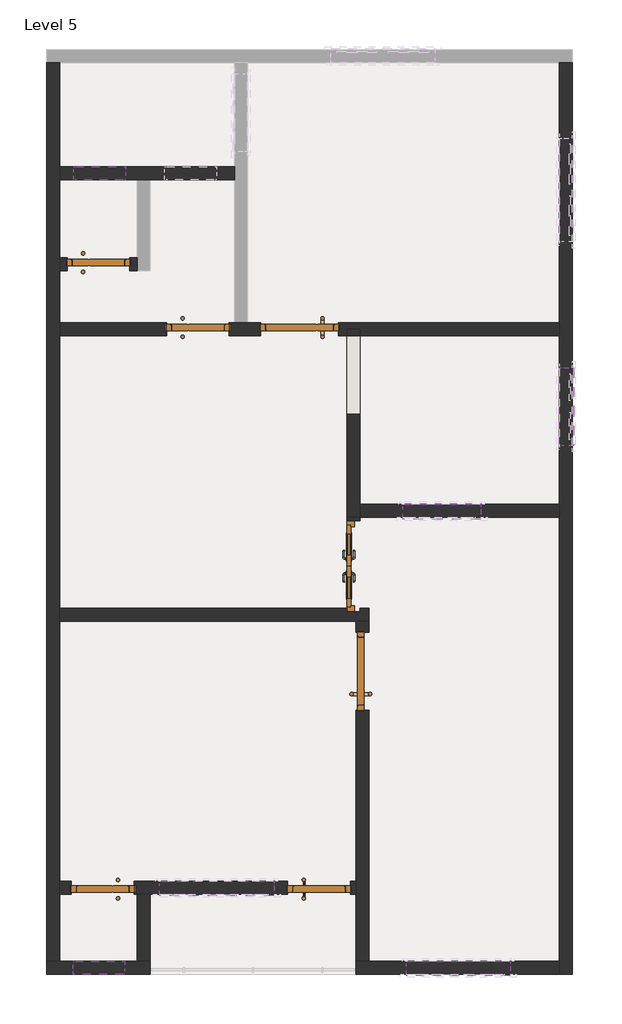
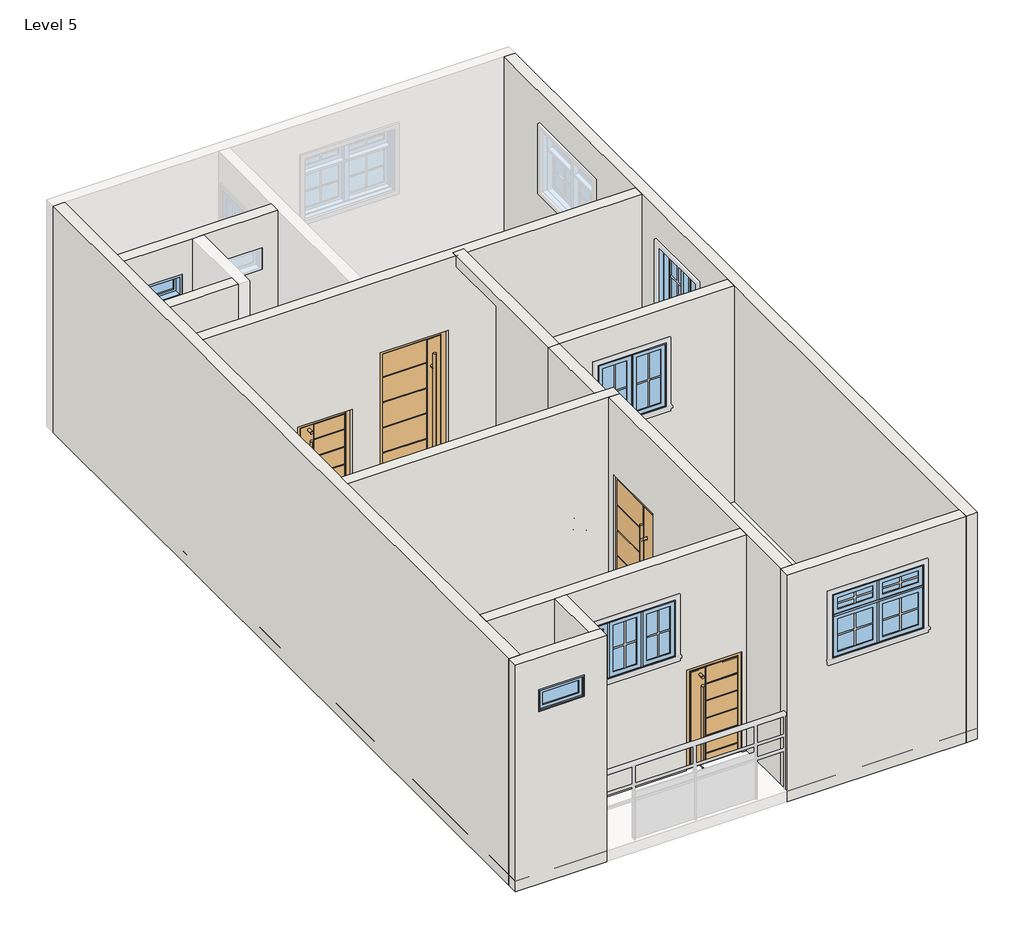
# One storey, part 1 of 2: 14 walls, 7 doors, 6 windows.
"""IFC4 building model written with IfcOpenShell, lengths in millimetres."""

from ifc_helpers import new_model, si_unit, frame, origin, place, context, project, spatial, polyline, outline, extrude, faceted_brep, transform, mapped, element, save
from components import door_9b787682, door_dc81b0c5, door_3_5c4206ef, door_3_79df91aa, door_2576ec39, door_55c03dfd, fixed_2_65c13adb, window_61697a4f, m_window_casement_double_3_e0bd8fa3, m_window_casement_double_awning_double_4_7efa9bbd

model = new_model("IFC4")

# Units and contexts
model_context = context("Model", 3, world=origin())
ifc_project = project(units=[si_unit("LENGTHUNIT", "METRE", prefix="MILLI")], contexts=[model_context])

# Site, building, storey
site = spatial("IfcSite", under=ifc_project)
building = spatial("IfcBuilding", under=site)
storey = spatial("IfcBuildingStorey", under=building, Name="Level 5", Elevation=3810.0)

# Doors
placement = place(None, origin())
door_shape = door_9b787682(model_context)
element("IfcDoor", 1, ObjectType="2'5\"", at=placement, inside=storey, context=model_context, shape_type="MappedRepresentation", body=[
    mapped(door_shape, transform((-22033.2963079, 3049.4742053, 3810.0), x_axis=(1.0, 0.0, 0.0), y_axis=(0.0, 1.0, 0.0), z_axis=(0.0, 0.0, 1.0))),
])
element("IfcDoor", 2, ObjectType="2'5\"", at=placement, inside=storey, context=model_context, shape_type="MappedRepresentation", body=[
    mapped(door_shape, transform((-23201.6963079, 3811.4742053, 3810.0), x_axis=(1.0, 0.0, 0.0), y_axis=(0.0, 1.0, 0.0), z_axis=(0.0, 0.0, 1.0))),
])
element("IfcDoor", 3, ObjectType="2'5\"", at=placement, inside=storey, context=model_context, shape_type="MappedRepresentation", body=[
    mapped(door_shape, transform((-23150.8963079, -3503.7257947, 3810.0), x_axis=(-1.0, 0.0, 0.0), y_axis=(0.0, -1.0, 0.0), z_axis=(0.0, 0.0, 1.0))),
])
door_2_shape = door_dc81b0c5(model_context)
element("IfcDoor", 4, ObjectType="2'5\"", at=placement, inside=storey, context=model_context, shape_type="MappedRepresentation", body=[
    mapped(door_2_shape, transform((-20610.8963079, -3503.7257947, 3856.2445349), x_axis=(1.0, 0.0, 0.0), y_axis=(0.0, 1.0, 0.0), z_axis=(0.0, 0.0, 1.0))),
])
door_3_shape = door_3_5c4206ef(model_context)
element("IfcDoor", 5, ObjectType="3'", at=placement, inside=storey, context=model_context, shape_type="MappedRepresentation", body=[
    mapped(door_3_shape, transform((-20102.8963079, -963.7257947, 3810.0), x_axis=(0.0, 1.0, 0.0), y_axis=(-1.0, 0.0, 0.0), z_axis=(0.0, 0.0, 1.0))),
])
door_3_2_shape = door_3_79df91aa(model_context)
element("IfcDoor", 6, ObjectType="3'", at=placement, inside=storey, context=model_context, shape_type="MappedRepresentation", body=[
    mapped(door_3_2_shape, transform((-20839.4963079, 3049.4742053, 3810.0), x_axis=(-1.0, 0.0, 0.0), y_axis=(0.0, -1.0, 0.0), z_axis=(0.0, 0.0, 1.0))),
])
door_4_shape = door_2576ec39(model_context)
door_5_shape = door_55c03dfd(model_context)
element("IfcDoor", 7, ObjectType="ExtDbl (8) : 3'6\"", at=placement, inside=storey, context=model_context, shape_type="MappedRepresentation", body=[
    mapped(door_4_shape, transform((-20204.4963079, 268.1742053, 3810.0), x_axis=(0.0, -1.0, 0.0), y_axis=(1.0, 0.0, 0.0), z_axis=(0.0, 0.0, 1.0))),
    mapped(door_5_shape, transform((-20204.4963079, 268.1742053, 3810.0), x_axis=(0.0, -1.0, 0.0), y_axis=(1.0, 0.0, 0.0), z_axis=(0.0, 0.0, 1.0))),
])

# Walls
element("IfcWall", 8, ObjectType="Generic - 6\"", at=placement, inside=storey, context=model_context, shape_type="Brep", body=[
    faceted_brep([(-17791.4963079, 6173.6742053, 3810.0), (-17791.4963079, 3125.6742053, 3810.0), (-17791.4963079, 2973.2742053, 3810.0), (-17791.4963079, 992.0742053, 3810.0), (-17791.4963079, 839.6742053, 3810.0), (-17791.4963079, -4367.3257947, 3810.0), (-17791.4963079, -4519.7257947, 3810.0), (-17791.4963079, -4519.7257947, 7010.4), (-17791.4963079, -4367.3257947, 7010.4), (-17791.4963079, 839.6742053, 7010.4), (-17791.4963079, 992.0742053, 7010.4), (-17791.4963079, 2973.2742053, 7010.4), (-17791.4963079, 3125.6742053, 7010.4), (-17791.4963079, 6173.6742053, 7010.4), (-17791.4963079, 4071.8242053, 6538.8), (-17791.4963079, 4071.8242053, 5638.8), (-17791.4963079, 5291.0242053, 5638.8), (-17791.4963079, 5291.0242053, 6538.8), (-17791.4963079, 1682.6367053, 6538.8), (-17791.4963079, 1682.6367053, 5638.8), (-17791.4963079, 2597.0367053, 5638.8), (-17791.4963079, 2597.0367053, 6538.8), (-17639.0963079, 6173.6742053, 3810.0), (-17639.0963079, 6173.6742053, 7010.4), (-17639.0963079, -4519.7257947, 7010.4), (-17639.0963079, -4519.7257947, 3810.0), (-17639.0963079, 4071.8242053, 6538.8), (-17639.0963079, 5291.0242053, 6538.8), (-17639.0963079, 5291.0242053, 5638.8), (-17639.0963079, 4071.8242053, 5638.8), (-17639.0963079, 1682.6367053, 6538.8), (-17639.0963079, 2597.0367053, 6538.8), (-17639.0963079, 2597.0367053, 5638.8), (-17639.0963079, 1682.6367053, 5638.8)], [[[0, 1, 2, 3, 4, 5, 6, 7, 8, 9, 10, 11, 12, 13], [14, 15, 16, 17], [18, 19, 20, 21]], [[22, 23, 24, 25], [26, 27, 28, 29], [30, 31, 32, 33]], [[6, 5, 4, 3, 2, 1, 0, 22, 25]], [[13, 12, 11, 10, 9, 8, 7, 24, 23]], [[0, 13, 23, 22]], [[7, 6, 25, 24]], [[15, 14, 26, 29]], [[16, 15, 29, 28]], [[17, 16, 28, 27]], [[14, 17, 27, 26]], [[19, 18, 30, 33]], [[20, 19, 33, 32]], [[21, 20, 32, 31]], [[18, 21, 31, 30]]]),
])
element("IfcWall", 9, ObjectType="Generic - 6\"", at=placement, inside=storey, context=model_context, shape_type="Brep", body=[
    faceted_brep([(-17791.4963079, -4367.3257947, 3810.0), (-20026.6963079, -4367.3257947, 3810.0), (-20179.0963079, -4367.3257947, 3810.0), (-20179.0963079, -4367.3257947, 7010.4), (-20026.6963079, -4367.3257947, 7010.4), (-17791.4963079, -4367.3257947, 7010.4), (-19585.5697454, -4367.3257947, 6538.8), (-19585.5697454, -4367.3257947, 5638.8), (-18366.3697454, -4367.3257947, 5638.8), (-18366.3697454, -4367.3257947, 6538.8), (-17791.4963079, -4519.7257947, 3810.0), (-17791.4963079, -4519.7257947, 7010.4), (-20179.0963079, -4519.7257947, 7010.4), (-20179.0963079, -4519.7257947, 3810.0), (-19585.5697454, -4519.7257947, 6538.8), (-18366.3697454, -4519.7257947, 6538.8), (-18366.3697454, -4519.7257947, 5638.8), (-19585.5697454, -4519.7257947, 5638.8)], [[[0, 1, 2, 3, 4, 5], [6, 7, 8, 9]], [[10, 11, 12, 13], [14, 15, 16, 17]], [[2, 1, 0, 10, 13]], [[5, 4, 3, 12, 11]], [[0, 5, 11, 10]], [[3, 2, 13, 12]], [[7, 6, 14, 17]], [[8, 7, 17, 16]], [[9, 8, 16, 15]], [[6, 9, 15, 14]]]),
])
element("IfcWall", 10, ObjectType="Generic - 6\"", at=placement, inside=storey, context=model_context, shape_type="Brep", body=[
    faceted_brep([(-23811.2963079, -4519.7257947, 3810.0), (-22592.0963079, -4519.7257947, 3810.0), (-22592.0963079, -4519.7257947, 7010.4), (-23811.2963079, -4519.7257947, 7010.4), (-23500.5431829, -4519.7257947, 6553.2), (-22890.9431829, -4519.7257947, 6553.2), (-22890.9431829, -4519.7257947, 6248.4), (-23500.5431829, -4519.7257947, 6248.4), (-23811.2963079, -4367.3257947, 3810.0), (-23811.2963079, -4367.3257947, 7010.4), (-23658.8963079, -4367.3257947, 7010.4), (-22744.4963079, -4367.3257947, 7010.4), (-22592.0963079, -4367.3257947, 7010.4), (-22592.0963079, -4367.3257947, 3810.0), (-22744.4963079, -4367.3257947, 3810.0), (-23658.8963079, -4367.3257947, 3810.0), (-23500.5431829, -4367.3257947, 6553.2), (-23500.5431829, -4367.3257947, 6248.4), (-22890.9431829, -4367.3257947, 6248.4), (-22890.9431829, -4367.3257947, 6553.2)], [[[0, 1, 2, 3], [4, 5, 6, 7]], [[8, 9, 10, 11, 12, 13, 14, 15], [16, 17, 18, 19]], [[1, 0, 8, 15, 14, 13]], [[3, 2, 12, 11, 10, 9]], [[0, 3, 9, 8]], [[2, 1, 13, 12]], [[17, 16, 4, 7]], [[18, 17, 7, 6]], [[19, 18, 6, 5]], [[16, 19, 5, 4]]]),
])
element("IfcWall", 11, ObjectType="Generic - 6\"", at=placement, inside=storey, context=model_context, shape_type="Brep", body=[
    faceted_brep([(-23658.8963079, -4367.3257947, 3810.0), (-23658.8963079, -3579.9257947, 3810.0), (-23658.8963079, -3427.5257947, 3810.0), (-23658.8963079, -379.5257947, 3810.0), (-23658.8963079, -227.1257947, 3810.0), (-23658.8963079, 2973.2742053, 3810.0), (-23658.8963079, 3125.6742053, 3810.0), (-23658.8963079, 3735.2742053, 3810.0), (-23658.8963079, 3887.6742053, 3810.0), (-23658.8963079, 4802.0742053, 3810.0), (-23658.8963079, 4954.4742053, 3810.0), (-23658.8963079, 6173.6742053, 3810.0), (-23658.8963079, 6173.6742053, 7010.4), (-23658.8963079, 4954.4742053, 7010.4), (-23658.8963079, 4802.0742053, 7010.4), (-23658.8963079, 3887.6742053, 7010.4), (-23658.8963079, 3735.2742053, 7010.4), (-23658.8963079, 3125.6742053, 7010.4), (-23658.8963079, 2973.2742053, 7010.4), (-23658.8963079, -227.1257947, 7010.4), (-23658.8963079, -379.5257947, 7010.4), (-23658.8963079, -3427.5257947, 7010.4), (-23658.8963079, -3579.9257947, 7010.4), (-23658.8963079, -4367.3257947, 7010.4), (-23811.2963079, -4367.3257947, 3810.0), (-23811.2963079, -4367.3257947, 7010.4), (-23811.2963079, 6173.6742053, 7010.4), (-23811.2963079, 6173.6742053, 3810.0)], [[[0, 1, 2, 3, 4, 5, 6, 7, 8, 9, 10, 11, 12, 13, 14, 15, 16, 17, 18, 19, 20, 21, 22, 23]], [[24, 25, 26, 27]], [[11, 10, 9, 8, 7, 6, 5, 4, 3, 2, 1, 0, 24, 27]], [[23, 22, 21, 20, 19, 18, 17, 16, 15, 14, 13, 12, 26, 25]], [[12, 11, 27, 26]], [[0, 23, 25, 24]]]),
])
element("IfcWall", 12, ObjectType="Generic - 6\"", at=placement, inside=storey, context=model_context, shape_type="Brep", body=[
    faceted_brep([(-17791.4963079, 2973.2742053, 7010.4), (-23658.8963079, 2973.2742053, 7010.4), (-23658.8963079, 2973.2742053, 3810.0), (-22401.5963079, 2973.2742053, 3810.0), (-22401.5963079, 2973.2742053, 5334.0), (-21664.9963079, 2973.2742053, 5334.0), (-21664.9963079, 2973.2742053, 3810.0), (-21296.6963079, 2973.2742053, 3810.0), (-21296.6963079, 2973.2742053, 5999.5), (-20382.2963079, 2973.2742053, 5999.5), (-20382.2963079, 2973.2742053, 3810.0), (-17791.4963079, 2973.2742053, 3810.0), (-23658.8963079, 3125.6742053, 7010.4), (-21601.4963079, 3125.6742053, 7010.4), (-21449.0963079, 3125.6742053, 7010.4), (-17791.4963079, 3125.6742053, 7010.4), (-17791.4963079, 3125.6742053, 3810.0), (-20382.2963079, 3125.6742053, 3810.0), (-20382.2963079, 3125.6742053, 5999.5), (-21296.6963079, 3125.6742053, 5999.5), (-21296.6963079, 3125.6742053, 3810.0), (-21449.0963079, 3125.6742053, 3810.0), (-21601.4963079, 3125.6742053, 3810.0), (-21664.9963079, 3125.6742053, 3810.0), (-21664.9963079, 3125.6742053, 5334.0), (-22401.5963079, 3125.6742053, 5334.0), (-22401.5963079, 3125.6742053, 3810.0), (-23658.8963079, 3125.6742053, 3810.0), (-22401.5963079, 3105.6742053, 3810.0), (-22416.5963079, 3105.6742053, 3810.0), (-22416.5963079, 3028.6742053, 3810.0), (-22401.5963079, 3028.6742053, 3810.0), (-20382.2963079, 3028.6742053, 3810.0), (-20367.2963079, 3028.6742053, 3810.0), (-20367.2963079, 3105.6742053, 3810.0), (-20382.2963079, 3105.6742053, 3810.0), (-21296.6963079, 3028.6742053, 3810.0), (-21664.9963079, 3028.6742053, 3810.0), (-21649.9963079, 3028.6742053, 3810.0), (-21649.9963079, 3105.6742053, 3810.0), (-21664.9963079, 3105.6742053, 3810.0), (-21296.6963079, 3105.6742053, 3810.0), (-21311.6963079, 3105.6742053, 3810.0), (-21311.6963079, 3028.6742053, 3810.0), (-21296.6963079, 3105.6742053, 5999.5), (-20382.2963079, 3105.6742053, 5999.5), (-20382.2963079, 3028.6742053, 5999.5), (-21296.6963079, 3028.6742053, 5999.5), (-21311.6963079, 3105.6742053, 6014.5), (-20367.2963079, 3105.6742053, 6014.5), (-20367.2963079, 3028.6742053, 6014.5), (-21311.6963079, 3028.6742053, 6014.5), (-21664.9963079, 3105.6742053, 5334.0), (-22401.5963079, 3105.6742053, 5334.0), (-22401.5963079, 3028.6742053, 5334.0), (-21664.9963079, 3028.6742053, 5334.0), (-22416.5963079, 3105.6742053, 5349.0), (-21649.9963079, 3105.6742053, 5349.0), (-21649.9963079, 3028.6742053, 5349.0), (-22416.5963079, 3028.6742053, 5349.0)], [[[0, 1, 2, 3, 4, 5, 6, 7, 8, 9, 10, 11]], [[12, 13, 14, 15, 16, 17, 18, 19, 20, 21, 22, 23, 24, 25, 26, 27]], [[2, 27, 26, 28, 29, 30, 31, 3]], [[16, 11, 10, 32, 33, 34, 35, 17]], [[36, 7, 6, 37, 38, 39, 40, 23, 22, 21, 20, 41, 42, 43]], [[1, 0, 15, 14, 13, 12]], [[0, 11, 16, 15]], [[2, 1, 12, 27]], [[44, 19, 18, 45]], [[46, 9, 8, 47]], [[19, 44, 41, 20]], [[47, 8, 7, 36]], [[45, 18, 17, 35]], [[9, 46, 32, 10]], [[48, 49, 50, 51]], [[48, 51, 43, 42]], [[46, 47, 36, 43, 51, 50, 33, 32]], [[50, 49, 34, 33]], [[44, 45, 35, 34, 49, 48, 42, 41]], [[24, 52, 53, 25]], [[4, 54, 55, 5]], [[52, 24, 23, 40]], [[5, 55, 37, 6]], [[25, 53, 28, 26]], [[54, 4, 3, 31]], [[56, 57, 58, 59]], [[58, 57, 39, 38]], [[55, 54, 31, 30, 59, 58, 38, 37]], [[56, 59, 30, 29]], [[53, 52, 40, 39, 57, 56, 29, 28]]]),
])
element("IfcWall", 13, ObjectType="Generic - 6\"", at=placement, inside=storey, context=model_context, shape_type="Brep", body=[
    faceted_brep([(-20280.6963079, 3049.4742053, 3810.0), (-20280.6963079, 839.6742053, 3810.0), (-20280.6963079, 839.6742053, 7010.4), (-20280.6963079, 3049.4742053, 7010.4), (-20280.6963079, 2974.7724011, 6858.0), (-20280.6963079, 2050.5574639, 6858.0), (-20280.6963079, 2050.5574639, 4419.6), (-20280.6963079, 2974.7724011, 4419.6), (-20128.2963079, 839.6742053, 3810.0), (-20128.2963079, 992.0742053, 3810.0), (-20128.2963079, 3049.4742053, 3810.0), (-20128.2963079, 3049.4742053, 7010.4), (-20128.2963079, 992.0742053, 7010.4), (-20128.2963079, 839.6742053, 7010.4), (-20128.2963079, 2050.5574639, 6858.0), (-20128.2963079, 2974.7724011, 6858.0), (-20128.2963079, 2974.7724011, 4419.6), (-20128.2963079, 2050.5574639, 4419.6)], [[[0, 1, 2, 3], [4, 5, 6, 7]], [[8, 9, 10, 11, 12, 13], [14, 15, 16, 17]], [[1, 0, 10, 9, 8]], [[3, 2, 13, 12, 11]], [[0, 3, 11, 10]], [[2, 1, 8, 13]], [[4, 15, 14, 5]], [[6, 17, 16, 7]], [[15, 4, 7, 16]], [[5, 14, 17, 6]]]),
])
element("IfcWall", 14, ObjectType="Generic - 6\"", at=placement, inside=storey, context=model_context, shape_type="SweptSolid", body=[
    extrude(outline(polyline([(3810.0, -20128.2963079), (3810.0, -17791.4963079), (7010.4, -17791.4963079), (7010.4, -20128.2963079), (3810.0, -20128.2963079)]), holes=[polyline([(6538.8, -19624.1658391), (6538.8, -18709.7658391), (5638.8, -18709.7658391), (5638.8, -19624.1658391), (6538.8, -19624.1658391)])]), frame((0.0, 839.6742053, 0.0), z_axis=(0.0, 1.0, 0.0), x_axis=(0.0, 0.0, 1.0)), (0.0, 0.0, 1.0), 152.4),
])
element("IfcWall", 15, ObjectType="Generic - 6\"", at=placement, inside=storey, context=model_context, shape_type="Brep", body=[
    faceted_brep([(-23658.8963079, -379.5257947, 3810.0), (-20179.0963079, -379.5257947, 3810.0), (-20026.6963079, -379.5257947, 3810.0), (-20026.6963079, -379.5257947, 7010.4), (-20179.0963079, -379.5257947, 7010.4), (-23658.8963079, -379.5257947, 7010.4), (-23658.8963079, -227.1257947, 7010.4), (-20280.6963079, -227.1257947, 7010.4), (-20128.2963079, -227.1257947, 7010.4), (-20026.6963079, -227.1257947, 7010.4), (-20026.6963079, -227.1257947, 3810.0), (-20128.2963079, -227.1257947, 3810.0), (-20128.2963079, -227.1257947, 5920.0), (-20280.6963079, -227.1257947, 5920.0), (-20280.6963079, -227.1257947, 3810.0), (-23658.8963079, -227.1257947, 3810.0), (-20280.6963079, -265.2257947, 3810.0), (-20128.2963079, -265.2257947, 3810.0), (-20280.6963079, -265.2257947, 5920.0), (-20128.2963079, -265.2257947, 5920.0)], [[[0, 1, 2, 3, 4, 5]], [[6, 7, 8, 9, 10, 11, 12, 13, 14, 15]], [[2, 1, 0, 15, 14, 16, 17, 11, 10]], [[5, 4, 3, 9, 8, 7, 6]], [[0, 5, 6, 15]], [[3, 2, 10, 9]], [[18, 16, 14, 13]], [[17, 19, 12, 11]], [[19, 18, 13, 12]], [[16, 18, 19, 17]]]),
])
element("IfcWall", 16, ObjectType="Generic - 6\"", at=placement, inside=storey, context=model_context, shape_type="Brep", body=[
    faceted_brep([(-20179.0963079, -4367.3257947, 7010.4), (-20179.0963079, -3579.9257947, 7010.4), (-20179.0963079, -3427.5257947, 7010.4), (-20179.0963079, -379.5257947, 7010.4), (-20179.0963079, -379.5257947, 3810.0), (-20179.0963079, -506.5257947, 3810.0), (-20179.0963079, -506.5257947, 5999.5), (-20179.0963079, -1420.9257947, 5999.5), (-20179.0963079, -1420.9257947, 3810.0), (-20179.0963079, -3427.5257947, 3810.0), (-20179.0963079, -3579.9257947, 3810.0), (-20179.0963079, -4367.3257947, 3810.0), (-20026.6963079, -379.5257947, 7010.4), (-20026.6963079, -4367.3257947, 7010.4), (-20026.6963079, -4367.3257947, 3810.0), (-20026.6963079, -1420.9257947, 3810.0), (-20026.6963079, -1420.9257947, 5999.5), (-20026.6963079, -506.5257947, 5999.5), (-20026.6963079, -506.5257947, 3810.0), (-20026.6963079, -379.5257947, 3810.0), (-20082.0963079, -506.5257947, 3810.0), (-20082.0963079, -491.5257947, 3810.0), (-20159.0963079, -491.5257947, 3810.0), (-20159.0963079, -506.5257947, 3810.0), (-20159.0963079, -1420.9257947, 3810.0), (-20159.0963079, -1435.9257947, 3810.0), (-20082.0963079, -1435.9257947, 3810.0), (-20082.0963079, -1420.9257947, 3810.0), (-20159.0963079, -506.5257947, 5999.5), (-20159.0963079, -1420.9257947, 5999.5), (-20082.0963079, -1420.9257947, 5999.5), (-20082.0963079, -506.5257947, 5999.5), (-20159.0963079, -1435.9257947, 6014.5), (-20159.0963079, -491.5257947, 6014.5), (-20082.0963079, -491.5257947, 6014.5), (-20082.0963079, -1435.9257947, 6014.5)], [[[0, 1, 2, 3, 4, 5, 6, 7, 8, 9, 10, 11]], [[12, 13, 14, 15, 16, 17, 18, 19]], [[4, 19, 18, 20, 21, 22, 23, 5]], [[14, 11, 10, 9, 8, 24, 25, 26, 27, 15]], [[3, 2, 1, 0, 13, 12]], [[0, 11, 14, 13]], [[4, 3, 12, 19]], [[6, 28, 29, 7]], [[16, 30, 31, 17]], [[28, 6, 5, 23]], [[17, 31, 20, 18]], [[7, 29, 24, 8]], [[30, 16, 15, 27]], [[32, 33, 34, 35]], [[34, 33, 22, 21]], [[31, 30, 27, 26, 35, 34, 21, 20]], [[32, 35, 26, 25]], [[29, 28, 23, 22, 33, 32, 25, 24]]]),
])
element("IfcWall", 17, ObjectType="Generic - 6\"", at=placement, inside=storey, context=model_context, shape_type="Brep", body=[
    faceted_brep([(-20179.0963079, -3579.9257947, 7010.4), (-22592.0963079, -3579.9257947, 7010.4), (-22744.4963079, -3579.9257947, 7010.4), (-23658.8963079, -3579.9257947, 7010.4), (-23658.8963079, -3579.9257947, 3810.0), (-23519.1963079, -3579.9257947, 3810.0), (-23519.1963079, -3579.9257947, 5334.0), (-22782.5963079, -3579.9257947, 5334.0), (-22782.5963079, -3579.9257947, 3810.0), (-22744.4963079, -3579.9257947, 3810.0), (-22592.0963079, -3579.9257947, 3810.0), (-20179.0963079, -3579.9257947, 3810.0), (-22484.1463079, -3579.9257947, 5638.8), (-22484.1463079, -3579.9257947, 6438.8), (-21137.9463079, -3579.9257947, 6438.8), (-21137.9463079, -3579.9257947, 5638.8), (-20979.1963079, -3579.9257947, 5380.2445349), (-20242.5963079, -3579.9257947, 5380.2445349), (-20242.5963079, -3579.9257947, 3856.2445349), (-20979.1963079, -3579.9257947, 3856.2445349), (-23658.8963079, -3427.5257947, 7010.4), (-20179.0963079, -3427.5257947, 7010.4), (-20179.0963079, -3427.5257947, 3810.0), (-22782.5963079, -3427.5257947, 3810.0), (-22782.5963079, -3427.5257947, 5334.0), (-23519.1963079, -3427.5257947, 5334.0), (-23519.1963079, -3427.5257947, 3810.0), (-23658.8963079, -3427.5257947, 3810.0), (-22484.1463079, -3427.5257947, 6438.8), (-22484.1463079, -3427.5257947, 5638.8), (-21137.9463079, -3427.5257947, 5638.8), (-21137.9463079, -3427.5257947, 6438.8), (-20242.5963079, -3427.5257947, 5380.2445349), (-20979.1963079, -3427.5257947, 5380.2445349), (-20979.1963079, -3427.5257947, 3856.2445349), (-20242.5963079, -3427.5257947, 3856.2445349), (-23519.1963079, -3482.9257947, 3810.0), (-23534.1963079, -3482.9257947, 3810.0), (-23534.1963079, -3559.9257947, 3810.0), (-23519.1963079, -3559.9257947, 3810.0), (-22782.5963079, -3559.9257947, 3810.0), (-22767.5963079, -3559.9257947, 3810.0), (-22767.5963079, -3482.9257947, 3810.0), (-22782.5963079, -3482.9257947, 3810.0), (-20979.1963079, -3559.9257947, 5380.2445349), (-20242.5963079, -3559.9257947, 5380.2445349), (-20242.5963079, -3482.9257947, 5380.2445349), (-20979.1963079, -3482.9257947, 5380.2445349), (-20242.5963079, -3559.9257947, 3856.2445349), (-20242.5963079, -3482.9257947, 3856.2445349), (-20227.5963079, -3559.9257947, 3856.2445349), (-20227.5963079, -3482.9257947, 3856.2445349), (-20979.1963079, -3482.9257947, 3856.2445349), (-20994.1963079, -3482.9257947, 3856.2445349), (-20994.1963079, -3559.9257947, 3856.2445349), (-20979.1963079, -3559.9257947, 3856.2445349), (-20994.1963079, -3559.9257947, 5395.2445349), (-20994.1963079, -3482.9257947, 5395.2445349), (-20227.5963079, -3482.9257947, 5395.2445349), (-20227.5963079, -3559.9257947, 5395.2445349), (-23519.1963079, -3559.9257947, 5334.0), (-22782.5963079, -3559.9257947, 5334.0), (-22782.5963079, -3482.9257947, 5334.0), (-23519.1963079, -3482.9257947, 5334.0), (-22767.5963079, -3559.9257947, 5349.0), (-23534.1963079, -3559.9257947, 5349.0), (-23534.1963079, -3482.9257947, 5349.0), (-22767.5963079, -3482.9257947, 5349.0)], [[[0, 1, 2, 3, 4, 5, 6, 7, 8, 9, 10, 11], [12, 13, 14, 15], [16, 17, 18, 19]], [[20, 21, 22, 23, 24, 25, 26, 27], [28, 29, 30, 31], [32, 33, 34, 35]], [[4, 27, 26, 36, 37, 38, 39, 5]], [[22, 11, 10, 9, 8, 40, 41, 42, 43, 23]], [[3, 2, 1, 0, 21, 20]], [[4, 3, 20, 27]], [[0, 11, 22, 21]], [[29, 28, 13, 12]], [[30, 29, 12, 15]], [[31, 30, 15, 14]], [[28, 31, 14, 13]], [[16, 44, 45, 17]], [[32, 46, 47, 33]], [[17, 45, 48, 18]], [[46, 32, 35, 49]], [[18, 48, 50, 51, 49, 35, 34, 52, 53, 54, 55, 19]], [[44, 16, 19, 55]], [[33, 47, 52, 34]], [[56, 57, 58, 59]], [[51, 50, 59, 58]], [[47, 46, 49, 51, 58, 57, 53, 52]], [[54, 53, 57, 56]], [[45, 44, 55, 54, 56, 59, 50, 48]], [[6, 60, 61, 7]], [[24, 62, 63, 25]], [[60, 6, 5, 39]], [[25, 63, 36, 26]], [[7, 61, 40, 8]], [[62, 24, 23, 43]], [[64, 65, 66, 67]], [[66, 65, 38, 37]], [[63, 62, 43, 42, 67, 66, 37, 36]], [[64, 67, 42, 41]], [[61, 60, 39, 38, 65, 64, 41, 40]]]),
])
element("IfcWall", 18, ObjectType="Generic - 6\"", at=placement, inside=storey, context=model_context, shape_type="SweptSolid", body=[
    extrude(outline(polyline([(-22744.4963079, -4367.3257947), (-22744.4963079, -3579.9257947), (-22592.0963079, -3579.9257947), (-22592.0963079, -4367.3257947), (-22744.4963079, -4367.3257947)])), frame((0.0, 0.0, 3810.0), z_axis=(0.0, 0.0, 1.0), x_axis=(1.0, 0.0, 0.0)), (0.0, 0.0, 1.0), 3200.4),
])
element("IfcWall", 19, ObjectType="Generic - 6\"", at=placement, inside=storey, context=model_context, shape_type="Brep", body=[
    faceted_brep([(-23658.8963079, 4802.0742053, 3810.0), (-22744.4963079, 4802.0742053, 3810.0), (-22592.0963079, 4802.0742053, 3810.0), (-21601.4963079, 4802.0742053, 3810.0), (-21601.4963079, 4802.0742053, 7010.4), (-22592.0963079, 4802.0742053, 7010.4), (-22744.4963079, 4802.0742053, 7010.4), (-23658.8963079, 4802.0742053, 7010.4), (-22880.5252141, 4802.0742053, 6553.2), (-22880.5252141, 4802.0742053, 6248.4), (-23490.1252141, 4802.0742053, 6248.4), (-23490.1252141, 4802.0742053, 6553.2), (-21812.6338079, 4802.0742053, 6553.2), (-21812.6338079, 4802.0742053, 6248.4), (-22422.2338079, 4802.0742053, 6248.4), (-22422.2338079, 4802.0742053, 6553.2), (-23658.8963079, 4954.4742053, 3810.0), (-23658.8963079, 4954.4742053, 7010.4), (-21601.4963079, 4954.4742053, 7010.4), (-21601.4963079, 4954.4742053, 3810.0), (-22880.5252141, 4954.4742053, 6553.2), (-23490.1252141, 4954.4742053, 6553.2), (-23490.1252141, 4954.4742053, 6248.4), (-22880.5252141, 4954.4742053, 6248.4), (-21812.6338079, 4954.4742053, 6553.2), (-22422.2338079, 4954.4742053, 6553.2), (-22422.2338079, 4954.4742053, 6248.4), (-21812.6338079, 4954.4742053, 6248.4)], [[[0, 1, 2, 3, 4, 5, 6, 7], [8, 9, 10, 11], [12, 13, 14, 15]], [[16, 17, 18, 19], [20, 21, 22, 23], [24, 25, 26, 27]], [[3, 2, 1, 0, 16, 19]], [[7, 6, 5, 4, 18, 17]], [[0, 7, 17, 16]], [[4, 3, 19, 18]], [[9, 8, 20, 23]], [[10, 9, 23, 22]], [[11, 10, 22, 21]], [[8, 11, 21, 20]], [[13, 12, 24, 27]], [[14, 13, 27, 26]], [[15, 14, 26, 25]], [[12, 15, 25, 24]]]),
])
element("IfcWall", 20, ObjectType="Generic - 6\"", at=placement, inside=storey, context=model_context, shape_type="Brep", body=[
    faceted_brep([(-22744.4963079, 3735.2742053, 7010.4), (-23658.8963079, 3735.2742053, 7010.4), (-23658.8963079, 3735.2742053, 3810.0), (-23569.9963079, 3735.2742053, 3810.0), (-23569.9963079, 3735.2742053, 5334.0), (-22833.3963079, 3735.2742053, 5334.0), (-22833.3963079, 3735.2742053, 3810.0), (-22744.4963079, 3735.2742053, 3810.0), (-23658.8963079, 3887.6742053, 7010.4), (-22744.4963079, 3887.6742053, 7010.4), (-22744.4963079, 3887.6742053, 3810.0), (-22833.3963079, 3887.6742053, 3810.0), (-22833.3963079, 3887.6742053, 5334.0), (-23569.9963079, 3887.6742053, 5334.0), (-23569.9963079, 3887.6742053, 3810.0), (-23658.8963079, 3887.6742053, 3810.0), (-23569.9963079, 3867.6742053, 3810.0), (-23584.9963079, 3867.6742053, 3810.0), (-23584.9963079, 3790.6742053, 3810.0), (-23569.9963079, 3790.6742053, 3810.0), (-22833.3963079, 3790.6742053, 3810.0), (-22818.3963079, 3790.6742053, 3810.0), (-22818.3963079, 3867.6742053, 3810.0), (-22833.3963079, 3867.6742053, 3810.0), (-22833.3963079, 3867.6742053, 5334.0), (-23569.9963079, 3867.6742053, 5334.0), (-23569.9963079, 3790.6742053, 5334.0), (-22833.3963079, 3790.6742053, 5334.0), (-23584.9963079, 3867.6742053, 5349.0), (-22818.3963079, 3867.6742053, 5349.0), (-22818.3963079, 3790.6742053, 5349.0), (-23584.9963079, 3790.6742053, 5349.0)], [[[0, 1, 2, 3, 4, 5, 6, 7]], [[8, 9, 10, 11, 12, 13, 14, 15]], [[2, 15, 14, 16, 17, 18, 19, 3]], [[10, 7, 6, 20, 21, 22, 23, 11]], [[1, 0, 9, 8]], [[0, 7, 10, 9]], [[2, 1, 8, 15]], [[12, 24, 25, 13]], [[4, 26, 27, 5]], [[24, 12, 11, 23]], [[5, 27, 20, 6]], [[13, 25, 16, 14]], [[26, 4, 3, 19]], [[28, 29, 30, 31]], [[30, 29, 22, 21]], [[27, 26, 19, 18, 31, 30, 21, 20]], [[28, 31, 18, 17]], [[25, 24, 23, 22, 29, 28, 17, 16]]]),
])
element("IfcWall", 21, ObjectType="Generic - 6\"", at=placement, inside=storey, context=model_context, shape_type="SweptSolid", body=[
    extrude(outline(polyline([(-227.1257947, 7010.4), (839.6742053, 7010.4), (839.6742053, 3810.0), (801.5742053, 3810.0), (801.5742053, 5920.0), (-227.1257947, 5920.0), (-227.1257947, 7010.4)])), frame((-20280.6963079, 0.0, 0.0), z_axis=(1.0, 0.0, 0.0), x_axis=(0.0, 1.0, 0.0)), (0.0, 0.0, 1.0), 152.4),
])

# Windows
fixed_2_shape = fixed_2_65c13adb(model_context)
element("IfcWindow", 22, ObjectType="Fixed : 2'", at=placement, inside=storey, context=model_context, shape_type="MappedRepresentation", body=[
    mapped(fixed_2_shape, transform((-23233.8431829, -4443.5257947, 5334.0), x_axis=(-1.0, 0.0, 0.0), y_axis=(0.0, -1.0, 0.0), z_axis=(0.0, 0.0, 1.0))),
])
element("IfcWindow", 23, ObjectType="Fixed : 2'", at=placement, inside=storey, context=model_context, shape_type="MappedRepresentation", body=[
    mapped(fixed_2_shape, transform((-23147.2252141, 4878.2742053, 5334.0), x_axis=(1.0, 0.0, 0.0), y_axis=(0.0, 1.0, 0.0), z_axis=(0.0, 0.0, 1.0))),
])
window_shape = window_61697a4f(model_context)
element("IfcWindow", 24, ObjectType="M_Window-Awning-Triple-Horizontal : 4'5\"", at=placement, inside=storey, context=model_context, shape_type="MappedRepresentation", body=[
    mapped(window_shape, transform((-21811.0463079, -3503.7257947, 4738.8), x_axis=(-1.0, 0.0, 0.0), y_axis=(0.0, -1.0, 0.0), z_axis=(0.0, 0.0, 1.0))),
])
m_window_casement_double_3_shape = m_window_casement_double_3_e0bd8fa3(model_context)
element("IfcWindow", 25, ObjectType="M_Window-Casement-Double : 3'", at=placement, inside=storey, context=model_context, shape_type="MappedRepresentation", body=[
    mapped(m_window_casement_double_3_shape, transform((-19166.9658391, 915.8742053, 4738.8), x_axis=(-1.0, 0.0, 0.0), y_axis=(0.0, -1.0, 0.0), z_axis=(0.0, 0.0, 1.0))),
])
element("IfcWindow", 26, ObjectType="M_Window-Casement-Double : 3'", at=placement, inside=storey, context=model_context, shape_type="MappedRepresentation", body=[
    mapped(m_window_casement_double_3_shape, transform((-17715.2963079, 2139.8367053, 4738.8), x_axis=(0.0, -1.0, 0.0), y_axis=(1.0, 0.0, 0.0), z_axis=(0.0, 0.0, 1.0))),
])
m_window_casement_double_awning_double_4_shape = m_window_casement_double_awning_double_4_7efa9bbd(model_context)
element("IfcWindow", 27, ObjectType="M_Window-Casement-Double-Awning-Double : 4'", at=placement, inside=storey, context=model_context, shape_type="MappedRepresentation", body=[
    mapped(m_window_casement_double_awning_double_4_shape, transform((-18975.9697454, -4443.5257947, 4738.8), x_axis=(-1.0, 0.0, 0.0), y_axis=(0.0, -1.0, 0.0), z_axis=(0.0, 0.0, 1.0))),
])

save(model, "model.ifc")

# Revit data of these elements
# Type "2'5\""
#   Type Mark = "9"
#   Water resistance = "up to Class E900, EN 12208:2001"
#   Uniclass2015Version = "v1.21"
#   Uniclass2015Reference = "Ss_25_30_20_30"
#   Uniclass2015Description = "Frame and door leaf system"
#   URL = "www.aluprof.com"
#   Type IFC Predefined Type = "USERDEFINED"
#   Right-hand / Left-hand door [instance default] = ""
#   Resistance to wind load = "up to Class C5/B5, EN 12210:2001"
#   Insert type = "ST"
#   Hardware [instance default] = ""
#   Product page = "https://aluprof.com/en/architects/offer/window-and-door-systems/panel-doors#visualisation"
#   Operation = "SinglePanelOutwardOpening"
#   Opening type = "Outward"
#   NBSReference = "25-50-20/125"
#   NBSDescription = "Frame and door leaf system"
#   Important = "The actual acceptable construction dimensions are dependent on the selection of profiles and hardware, glazing type, construction weight and the construction’s operating conditions. These should be determined by a suitably qualified person, and using ALUPROF’s calculation software"
#   IfcExportType = "USERDEFINED"
#   IfcExportAs = "IfcDoorType"
#   Handle type [instance default] = ""
#   Manufacturer = "ALUPROF SA"
#   Export Type to IFC As = "IfcDoorType"
#   Door sill type [instance default] = ""
#   Description = "External single-leaf panel door outward opening"
#   Model = "MB-86 ST Panel Door AD07"
#   Content of the recyclate in the material = "69.2%"
#   COBie.Type.WarrantyDurationParts = ""
#   COBie.Type.Name = ""
#   COBie.Type.Manufacturer = "ALUPROF SA"
#   COBie.Space.Name = ""
#   COBie.Floor.Name = ""
#   COBie.Facility.Name = ""
#   COBie.CreatedOn = ""
#   COBie.Component.WarrantyStartDate = ""
#   COBie.Component.Name = "MB-86 ST Panel Door AD07"
#   Burglar resistance = "RC2"
#   Air permeability = "up to Class 4, EN 12207:2001"
#   Width of the active leaf = 2' - 1.17717"
#   Placement in wall = 0' - 0.7874"
#   Thickness = 0' - 3.0315"
#   Height of the opening sash = 4' - 9.44094"
#   Handle Offset = 3' - 5.33858"
#   Rough Height = 5' - 2.40945"
#   Rough Width = 2' - 6.1811"
#   Height = 5' - 0"
#   Width = 2' - 5"
#   Construction depth = 0' - 3.0315"
#   Clear opening width = 1' - 8.94882"
#   Clear opening height = 4' - 8.47638"
#   Height of the array = 0' - 9.08136"
#   Schedule No. [instance default] = 1
#   Handrail [instance default] = yes
#   IsExternal = yes
#   Handle [instance default] = no
#   Door closer [instance default] = no
#   Function = 1
#   COBie.Type = yes
#   COBie = yes
#   Access control [instance default] = no
#   Panel = element 346771
#   Wall Closure = (empty or 0)
# Type "3'"
#   Type Mark = "10"
#   Water resistance = "up to Class E900, EN 12208:2001"
#   Uniclass2015Version = "v1.21"
#   Uniclass2015Reference = "Ss_25_30_20_30"
#   Uniclass2015Description = "Frame and door leaf system"
#   URL = "www.aluprof.com"
#   Type IFC Predefined Type = "USERDEFINED"
#   Right-hand / Left-hand door [instance default] = ""
#   Resistance to wind load = "up to Class C5/B5, EN 12210:2001"
#   Insert type = "ST"
#   Hardware [instance default] = ""
#   Product page = "https://aluprof.com/en/architects/offer/window-and-door-systems/panel-doors#visualisation"
#   Operation = "SinglePanelOutwardOpening"
#   Opening type = "Outward"
#   NBSReference = "25-50-20/125"
#   NBSDescription = "Frame and door leaf system"
#   Important = "The actual acceptable construction dimensions are dependent on the selection of profiles and hardware, glazing type, construction weight and the construction’s operating conditions. These should be determined by a suitably qualified person, and using ALUPROF’s calculation software"
#   IfcExportType = "USERDEFINED"
#   IfcExportAs = "IfcDoorType"
#   Handle type [instance default] = ""
#   Manufacturer = "ALUPROF SA"
#   Export Type to IFC As = "IfcDoorType"
#   Door sill type [instance default] = ""
#   Description = "External single-leaf panel door outward opening"
#   Model = "MB-86 ST Panel Door AD07"
#   Content of the recyclate in the material = "69.2%"
#   COBie.Type.WarrantyDurationParts = ""
#   COBie.Type.Name = ""
#   COBie.Type.Manufacturer = "ALUPROF SA"
#   COBie.Space.Name = ""
#   COBie.Floor.Name = ""
#   COBie.Facility.Name = ""
#   COBie.CreatedOn = ""
#   COBie.Component.WarrantyStartDate = ""
#   COBie.Component.Name = "MB-86 ST Panel Door AD07"
#   Burglar resistance = "RC2"
#   Air permeability = "up to Class 4, EN 12207:2001"
#   Width of the active leaf = 2' - 8.17717"
#   Placement in wall = 0' - 0.7874"
#   Thickness = 0' - 3.0315"
#   Height of the opening sash = 6' - 11.64173"
#   Handle Offset = 3' - 5.33858"
#   Rough Height = 7' - 4.61024"
#   Rough Width = 3' - 1.1811"
#   Height = 7' - 2.20079"
#   Width = 3' - 0"
#   Construction depth = 0' - 3.0315"
#   Clear opening width = 2' - 3.94882"
#   Clear opening height = 6' - 10.67717"
#   Height of the array = 1' - 1.44816"
#   Schedule No. [instance default] = 1
#   Handrail [instance default] = yes
#   IsExternal = yes
#   Handle [instance default] = no
#   Door closer [instance default] = no
#   Function = 1
#   COBie.Type = yes
#   COBie = yes
#   Access control [instance default] = no
#   Panel = element 346771
#   Wall Closure = (empty or 0)
# Type "ExtDbl (8) : 3'6\""
#   Type Mark = "14"
#   Operation = "DoubleDoorSingleSwing"
#   Keynote = "L20"
#   Wrap Layers (Int) from Ext = 0' - 6.98819"
#   Wrap Layers (Ext) from Ext = 0' - 4.03543"
#   Top of Lock Rail = 2' - 11.43307"
#   Thickness = 0' - 1.73228"
#   Stile Shutting = 0' - 4.92126"
#   Stile - Top Rail = 0' - 5.90551"
#   Stile - Lock Rail = 0' - 5.90551"
#   Stile - Hanging = 0' - 3.93701"
#   Stile - Bottom Rail = 0' - 11.81102"
#   Rough Width = 3' - 6"
#   Rough Height = 6' - 11.07087"
#   O/A Frame Width = 0' - 2.51969"
#   Handle Z Distance = 3' - 1.40157"
#   Glazing Thickness = 0' - 0.94488"
#   FrameWidth = 0' - 1.65354"
#   FrameOffset - External = 0' - 2.55906"
#   FrameDepth = 0' - 3.50394"
#   Door Panel Width = 1' - 6.91339"
#   Door Panel Thickness = 0' - 1.73228"
#   Door Panel Height = 6' - 6.74016"
#   Cill Thickness = 0' - 2.14567"
#   Cill Projection = 0' - 1.1811"
#   Handle X Distance = 0' - 2.95276"
#   Height = 6' - 11.07087"
#   Structural Tolerance = 0' - 0.25591"
#   Tolerance = 0' - 0.11811"
#   Undercut = 0' - 0.15748"
#   Width = 3' - 6"
#   Cill Extension = 0' - 0.98425"
#   Cavity Closer Width = 0' - 1.9685"
#   Cavity Closer Offset from Ext = 0' - 4.03543"
#   Cavity Closer Depth = 0' - 3.34646"
#   Vis - Ironmongery = yes
#   Vis - Cavity Closers = yes
#   Function = 1
#   Material Glass = Door - Glazing
#   Handle Style = element 349788
#   Material Door = Door - Panel
#   Material Ironmongery = Door - Handle
#   Wall Closure = (empty or 0)
# Type "Generic - 6\""
#   Assembly Code = "B2010"
#   Layers, outside or top first: 0' - 6" no material (function 1)
# Type "Fixed : 2'"
#   Type Mark = "16"
#   Assembly Code = "B2020100"
#   Height = 1' - 0"
#   Default Sill Height = 3' - 0"
#   Width = 2' - 0"
#   Window Inset = 0' - 0 3/4"
#   Glass Pane Material = Glass
#   Sash Material = Sash
#   Wall Closure = (empty or 0)
# Type "M_Window-Awning-Triple-Horizontal : 4'5\""
#   Type Mark = "15"
#   Fire Rating = "0.5h"
#   Assembly Code = "B2020100"
#   Analytic Construction = "Double glazing - domestic"
#   Window Inset [instance default] = 0' - 0"
#   Wall Thickness [instance default] = 0' - 5.90551"
#   Muntin Width = 1' - 0.33333"
#   Visual Light Transmittance = 0.81
#   Thermal Resistance (R) = 1.8146 (h·ft²·°F)/BTU
#   Solar Heat Gain Coefficient = 0.76
#   One Third Width = 1' - 5.66667"
#   Sash Width = 1' - 4.83333"
#   Rough Width = 4' - 5.59055"
#   Rough Height = 2' - 8.08661"
#   Interior Wall Closure [instance default] = 0' - 2.15551"
#   Height = 2' - 7.49606"
#   Heat Transfer Coefficient (U) = 0.5511 BTU/(h·ft²·°F)
#   Muntin Height = 2' - 1.99606"
#   Frame Extension [instance default] = 0' - 0 1/4"
#   Exterior Wall Closure [instance default] = 0' - 1 1/4"
#   Extension Jamb [instance default] = 0' - 2.15551"
#   Default Sill Height = 2' - 11.43307"
#   Width = 4' - 5"
#   Middle Muntin Visibility = yes
#   Side Muntin Visibility = yes
#   Interior Trim Visibility [instance default] = yes
#   Exterior Trim Visibility [instance default] = yes
#   Extension Jamb Visibility [instance default] = yes
#   Muntin Pattern = M_Muntin Pattern_2x2 : M_Muntin Pattern_2x2
#   Interior Trim Material = Wood - Stained
#   Interior Trim = M_Trim-Window-Interior-Flat : Picture Frame
#   Interior Frame Material = Wood - Stained
#   Glass Panel Material = Glass
#   Exterior Trim Material = Clad - White
#   Exterior Trim = M_Trim-Window-Exterior-Flat : with Sill
#   Exterior Frame Material = Clad - White
#   Wall Closure = (empty or 0)
# Type "M_Window-Casement-Double : 3'"
#   Type Mark = "13"
#   Fire Rating = "0.5h"
#   Assembly Code = "B2020100"
#   Analytic Construction = "Double glazing - domestic"
#   Frame Extension [instance default] = 0' - 0 1/4"
#   Window Inset [instance default] = 0' - 0"
#   Wall Thickness [instance default] = 0' - 5.90551"
#   Interior Wall Closure [instance default] = 0' - 2.15551"
#   Half Width = 1' - 6"
#   Visual Light Transmittance = 0.81
#   Thermal Resistance (R) = 1.8146 (h·ft²·°F)/BTU
#   Solar Heat Gain Coefficient = 0.76
#   Rough Width = 3' - 0.59055"
#   Rough Height = 3' - 0.02362"
#   Height = 2' - 11.43307"
#   Heat Transfer Coefficient (U) = 0.5511 BTU/(h·ft²·°F)
#   Exterior Wall Closure [instance default] = 0' - 1.25197"
#   Extension Jamb [instance default] = 0' - 2.15551"
#   Default Sill Height = 2' - 11.43307"
#   Width = 3' - 0"
#   Muntin Visibility = yes
#   Interior Trim Visibility [instance default] = yes
#   Exterior Trim Visibility [instance default] = yes
#   Extension Jamb Visibility [instance default] = yes
#   Interior Trim Material = Wood - Stained
#   Muntin Pattern = M_Muntin Pattern_2x2 : M_Muntin Pattern_2x2
#   Interior Trim = M_Trim-Window-Interior-Flat : Picture Frame
#   Interior Frame Material = Wood - Stained
#   Glass Panel Material = Glass
#   Exterior Trim Material = Clad - White
#   Exterior Trim = M_Trim-Window-Exterior-Flat : with Sill
#   Exterior Frame Material = Clad - White
#   Wall Closure = (empty or 0)
# Type "M_Window-Casement-Double-Awning-Double : 4'"
#   Type Mark = "11"
#   Fire Rating = "0.5h"
#   Assembly Code = "B2020100"
#   Analytic Construction = "Double glazing - domestic"
#   Window Inset [instance default] = 0' - 0"
#   Wall Thickness [instance default] = 0' - 5.90551"
#   Interior Wall Closure [instance default] = 0' - 2.15551"
#   Half Width = 2' - 0"
#   Visual Light Transmittance = 0.81
#   Transom Height = 0' - 11.81102"
#   Thermal Resistance (R) = 1.8146 (h·ft²·°F)/BTU
#   Solar Heat Gain Coefficient = 0.76
#   Rough Width = 4' - 0.59055"
#   Rough Height = 3' - 0.02362"
#   Open Window Height = 1' - 11.62205"
#   Frame Extension [instance default] = 0' - 0 1/4"
#   Height = 2' - 11.43307"
#   Heat Transfer Coefficient (U) = 0.5511 BTU/(h·ft²·°F)
#   Exterior Wall Closure [instance default] = 0' - 1.25197"
#   Extension Jamb [instance default] = 0' - 2.15551"
#   Default Sill Height = 2' - 11.43307"
#   Width = 4' - 0"
#   Top Muntin Visibility = yes
#   Bottom Muntin Visibility = yes
#   Interior Trim Visibility [instance default] = yes
#   Exterior Trim Visibility [instance default] = yes
#   Extension Jamb Visibility [instance default] = yes
#   Interior Trim Material = Wood - Stained
#   Muntin Pattern = M_Muntin Pattern_2x2 : M_Muntin Pattern_2x2
#   Interior Trim = M_Trim-Window-Interior-Flat : Picture Frame
#   Interior Frame Material = Wood - Stained
#   Glass Panel Material = Glass
#   Exterior Trim Material = Clad - White
#   Exterior Trim = M_Trim-Window-Exterior-Flat : with Sill
#   Exterior Frame Material = Clad - White
#   Wall Closure = (empty or 0)
# Elements 1, 2, 3, 4 (IfcDoor, "2'5\"")
#   Right-hand / Left-hand door = ""
#   Hardware = ""
#   Handle type = ""
#   Door sill type = ""
#   Schedule No. = 1
#   Handrail = yes
#   Handle = no
#   Door closer = no
#   Access control = no
#   Phase Created = New Construction
# Elements 5, 6 (IfcDoor, "3'")
#   Right-hand / Left-hand door = ""
#   Hardware = ""
#   Handle type = ""
#   Door sill type = ""
#   Schedule No. = 1
#   Handrail = yes
#   Handle = no
#   Door closer = no
#   Access control = no
#   Phase Created = New Construction
# Element 7 (IfcDoor, "ExtDbl (8) : 3'6\"")
#   Phase Created = New Construction
#   Materials on its faces: "Door - Panel", "Door - Handle", "Door - Glazing"
# Elements 8, 9, 10, 11 (IfcWall, "Generic - 6\"")
#   Top Offset = 0' - 0"
#   Base Offset = 0' - 0"
#   Unconnected Height = 10' - 6"
#   wall height = 10' - 6"
#   Phase Created = New Construction
#   Base Constraint = Level 5
#   Materials on its faces: "Default Wall", "Parking Stripe"
# Elements 12, 13, 14, 15, 16, 17, 18, 19, 20, 21 (IfcWall, "Generic - 6\"")
#   Top Offset = 0' - 0"
#   Base Offset = 0' - 0"
#   Unconnected Height = 10' - 6"
#   wall height = 10' - 6"
#   Phase Created = New Construction
#   Base Constraint = Level 5
#   Materials on its faces: "Default Wall"
# Element 22 (IfcWindow, "Fixed : 2'")
#   Mark = "18"
#   Phase Created = New Construction
#   Materials on its faces: "Sash", "Glass"
# Element 23 (IfcWindow, "Fixed : 2'")
#   Mark = "19"
#   Phase Created = New Construction
#   Materials on its faces: "Sash", "Glass"
# Element 24 (IfcWindow, "M_Window-Awning-Triple-Horizontal : 4'5\"")
#   Mark = "17"
#   Window Inset = 0' - 0"
#   Interior Wall Closure = 0' - 2.15551"
#   Frame Extension = 0' - 0 1/4"
#   Exterior Wall Closure = 0' - 1 1/4"
#   Interior Trim Visibility = yes
#   Exterior Trim Visibility = yes
#   Phase Created = New Construction
#   Materials on its faces: "Wood - Stained", "Glass", "Clad - White"
# Element 25 (IfcWindow, "M_Window-Casement-Double : 3'")
#   Mark = "14"
#   Window Inset = 0' - 0"
#   Interior Wall Closure = 0' - 2.15551"
#   Frame Extension = 0' - 0 1/4"
#   Exterior Wall Closure = 0' - 1.25197"
#   Interior Trim Visibility = yes
#   Exterior Trim Visibility = yes
#   Phase Created = New Construction
#   Materials on its faces: "Wood - Stained", "Glass", "Clad - White"
# Element 26 (IfcWindow, "M_Window-Casement-Double : 3'")
#   Mark = "15"
#   Window Inset = 0' - 0"
#   Interior Wall Closure = 0' - 2.15551"
#   Frame Extension = 0' - 0 1/4"
#   Exterior Wall Closure = 0' - 1.25197"
#   Interior Trim Visibility = yes
#   Exterior Trim Visibility = yes
#   Phase Created = New Construction
#   Materials on its faces: "Wood - Stained", "Glass", "Clad - White"
# Element 27 (IfcWindow, "M_Window-Casement-Double-Awning-Double : 4'")
#   Mark = "13"
#   Window Inset = 0' - 0"
#   Interior Wall Closure = 0' - 2.15551"
#   Frame Extension = 0' - 0 1/4"
#   Exterior Wall Closure = 0' - 1.25197"
#   Interior Trim Visibility = yes
#   Exterior Trim Visibility = yes
#   Phase Created = New Construction
#   Materials on its faces: "Wood - Stained", "Glass", "Clad - White"
# Materials
#   "Door - Glazing": colour RGB 0 0 255, transparency 0.75
#   "Door - Panel": class "Wood", colour RGB 114 82 51, transparency 0
#   "Door - Handle": colour RGB 247 247 247, transparency 0
#   "Glass": class "Glass", colour RGB 218 227 224, transparency 0.85, Description = "Soda Lime Glass", Cost = 0
#   "Sash": class "Wood", colour RGB 136 99 55, transparency 0
#   "Wood - Stained": class "Wood", colour RGB 227 170 128, transparency 0, Cost = 0
#   "Clad - White": class "Wood", colour RGB 242 242 238, transparency 0, Cost = 0
#   "Default Wall": colour RGB 80 80 80, transparency 0
#   "Parking Stripe": class "Paint", colour RGB 226 219 42, transparency 0
